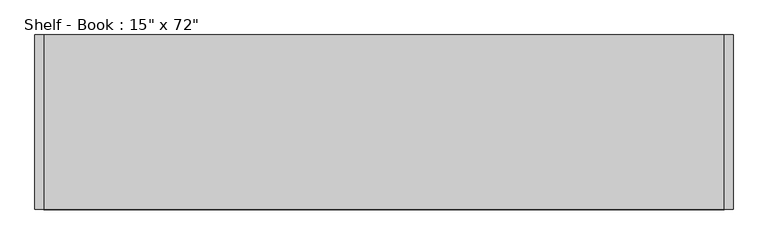
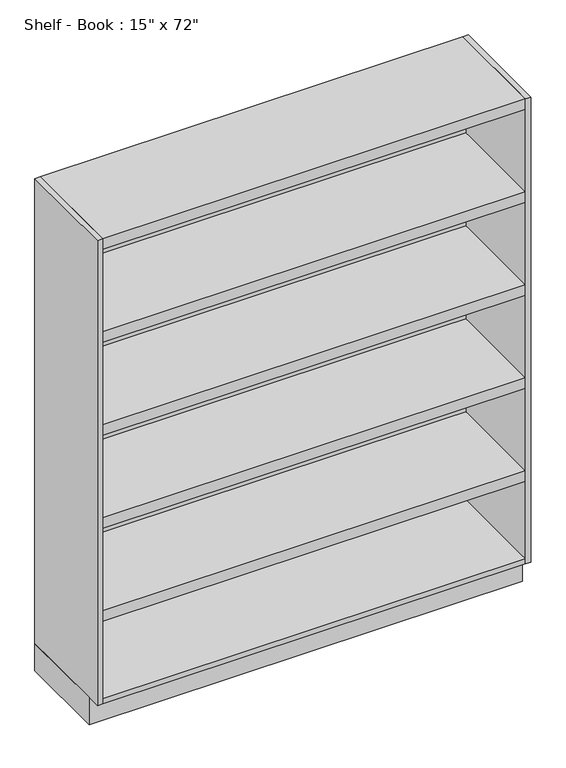
"""IFC4 building model written with IfcOpenShell, lengths in millimetres: proxy geometry."""

from ifc_helpers import new_model, si_unit, frame, origin, origin_with_axes, place, context, project, spatial, polyline, outline, extrude, source, transform, mapped, element, save


def proxy_420707f7(model_context):
    return source(origin(), model_context, "Body", "SweptSolid", [
        extrude(outline(polyline([(1524.0, 0.0), (1524.0, -330.2), (0.0, -330.2), (0.0, 0.0), (1524.0, 0.0)])), origin_with_axes(), (0.0, 0.0, 1.0), 101.6),
        extrude(outline(polyline([(19.05, 0.0), (19.05, -381.0), (0.0, -381.0), (0.0, 0.0), (19.05, 0.0)])), frame((0.0, 0.0, 101.6), z_axis=(0.0, 0.0, 1.0), x_axis=(1.0, 0.0, 0.0)), (0.0, 0.0, 1.0), 1727.2),
        extrude(outline(polyline([(1504.95, 0.0), (1524.0, 0.0), (1524.0, -381.0), (1504.95, -381.0), (1504.95, 0.0)])), frame((0.0, 0.0, 101.6), z_axis=(0.0, 0.0, 1.0), x_axis=(1.0, 0.0, 0.0)), (0.0, 0.0, 1.0), 1727.2),
        extrude(outline(polyline([(-381.0, 101.6), (-381.0, 120.65), (-19.05, 120.65), (-19.05, 427.99), (-361.95, 427.99), (-361.95, 408.94), (-381.0, 408.94), (-381.0, 447.04), (-19.05, 447.04), (-19.05, 773.43), (-361.95, 773.43), (-361.95, 754.38), (-381.0, 754.38), (-381.0, 792.48), (-19.05, 792.48), (-19.05, 1118.87), (-361.95, 1118.87), (-361.95, 1099.82), (-381.0, 1099.82), (-381.0, 1137.92), (-19.05, 1137.92), (-19.05, 1464.31), (-361.95, 1464.31), (-361.95, 1445.26), (-381.0, 1445.26), (-381.0, 1483.36), (-19.05, 1483.36), (-19.05, 1809.75), (-361.95, 1809.75), (-361.95, 1790.7), (-381.0, 1790.7), (-381.0, 1828.8), (0.0, 1828.8), (0.0, 101.6), (-381.0, 101.6)])), frame((19.05, 0.0, 0.0), z_axis=(1.0, 0.0, 0.0), x_axis=(0.0, 1.0, 0.0)), (0.0, 0.0, 1.0), 1485.9),
    ])


if __name__ == "__main__":
    model = new_model("IFC4")
    model_context = context("Model", 3, world=origin())
    ifc_project = project(units=[si_unit("LENGTHUNIT", "METRE", prefix="MILLI")], contexts=[model_context])
    site = spatial("IfcSite", under=ifc_project)
    building = spatial("IfcBuilding", under=site)
    placement = place(None, origin())
    proxy_shape = proxy_420707f7(model_context)
    element("IfcBuildingElementProxy", 1, Name="Shelf - Book : 15\" x 72\"", ObjectType="Shelf - Book : 15\" x 72\"", at=placement, inside=building, context=model_context, shape_type="MappedRepresentation", body=[
        mapped(proxy_shape, transform((0.0, 0.0, 0.0), x_axis=(1.0, 0.0, 0.0), y_axis=(0.0, 1.0, 0.0), z_axis=(0.0, 0.0, 1.0))),
    ])
    save(model, "model.ifc")

# Revit data of these elements
# Type "Shelf - Book : 15\" x 72\""
#   Assembly Code = "E1010510"
#   Depth = 381 mm
#   Height = 1828.8 mm
#   Length [instance default] = 1524 mm
#   Base Material = Finishes - Paint - Black
#   Material = Laminate - Ivory,Matte
#   Default Elevation = 0
# Element 1 (IfcBuildingElementProxy, "Shelf - Book : 15\" x 72\"")
#   Materials on its faces: "Laminate - Ivory,Matte", "Finishes - Paint - Black"
# Materials
#   "Finishes - Paint - Black": colour RGB 0 0 0, transparency 0
#   "Laminate - Ivory,Matte": colour RGB 247 247 239, transparency 0
